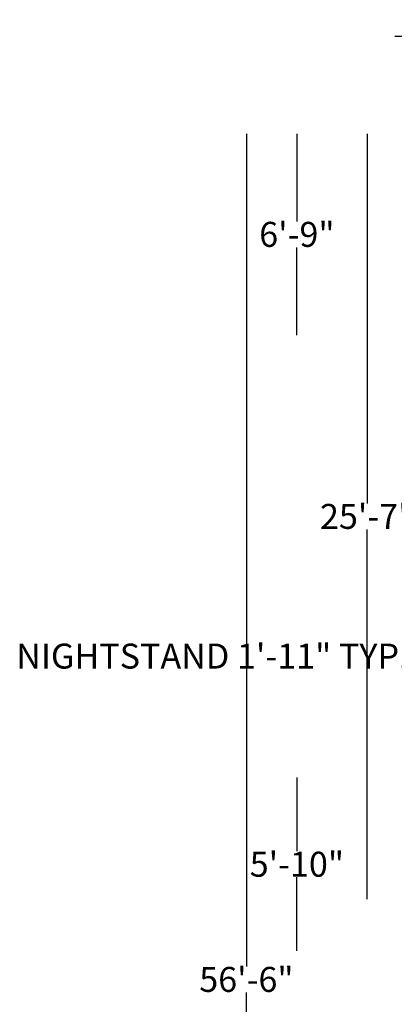
# Model space of a CAD drawing. Units: inches. Extents: x 1198 to 8596, y 144 to 930.
# Tile 2 of 5: x 1198 to 1348, y 536 to 930. Entities that reach past the tile are written whole.
import ezdxf

# ---------------------------------------------------------------- set-up
doc = ezdxf.new("R2010")
doc.units = ezdxf.units.IN
doc.header["$MEASUREMENT"] = 0
doc.layers.add('A-ANNO-DIMS', color=7, linetype='Continuous', lineweight=18)
doc.styles.get("Standard").update_dxf_attribs({"font": 'arial.ttf'})
doc.dimstyles.get("Standard").update_dxf_attribs({"dimtxt": 10, "dimasz": 0.18, "dimexe": 0.18, "dimexo": 0.0625, "dimgap": 0.09, "dimtad": 0, "dimtih": 1, "dimtoh": 1, "dimdec": 0, "dimzin": 0, "dimdsep": 46, "dimlunit": 3, "dimtxsty": 'Standard', "dimcen": 0.09, "dimse1": 1, "dimse2": 1, "dimadec": 0, "dimazin": 0, "dimtfac": 1, "dimtdec": 0, "dimtofl": 0, "dimtmove": 0, "dimatfit": 3, "dimfxl": 1, "dimtolj": 1, "dimtzin": 0, "dimarcsym": 0})

# ---------------------------------------------------------------- blocks, each defined once
blk = doc.blocks.new('*D16')
at = {"layer": 'A-ANNO-DIMS', "color": 0, "lineweight": -2, "transparency": 16777216}
for p, q in [((1337.03, 884.72), (1337.03, 736.59)), ((1337.03, 578.08), (1337.03, 726.2))]:
    blk.add_line(p, q, dxfattribs=at)
at = {"layer": 'A-ANNO-DIMS', "color": 0, "transparency": 16777216}
for points in [[(1337, 884.72), (1337.06, 884.72), (1337.03, 884.9)], [(1337, 578.08), (1337.06, 578.08), (1337.03, 577.9)]]:
    blk.add_solid(points, dxfattribs=at)
at = {"layer": 'Defpoints', "color": 0, "transparency": 16777216}
for p in [(1347.89, 884.9), (1337.03, 577.9), (1347.89, 577.9)]:
    blk.add_point(p, dxfattribs=at)
at = {"layer": 'A-ANNO-DIMS', "color": 0, "transparency": 16777216, "insert": (1337.03, 731.4), "char_height": 10, "attachment_point": 5}
blk.add_mtext('\\A1;25\'-7"', dxfattribs=at)
blk = doc.blocks.new('*D17')
at = {"layer": 'A-ANNO-DIMS', "color": 0, "lineweight": -2, "transparency": 16777216}
for p, q in [((1288.75, 884.72), (1288.75, 551.09)), ((1288.75, 207.08), (1288.75, 540.7))]:
    blk.add_line(p, q, dxfattribs=at)
at = {"layer": 'A-ANNO-DIMS', "color": 0, "transparency": 16777216}
for points in [[(1288.72, 884.72), (1288.78, 884.72), (1288.75, 884.9)], [(1288.72, 207.08), (1288.78, 207.08), (1288.75, 206.9)]]:
    blk.add_solid(points, dxfattribs=at)
at = {"layer": 'Defpoints', "color": 0, "transparency": 16777216}
for p in [(1347.89, 884.9), (1288.75, 206.9), (1347.89, 206.9)]:
    blk.add_point(p, dxfattribs=at)
at = {"layer": 'A-ANNO-DIMS', "color": 0, "transparency": 16777216, "insert": (1288.75, 545.9), "char_height": 10, "attachment_point": 5}
blk.add_mtext('\\A1;56\'-6"', dxfattribs=at)
blk = doc.blocks.new('*D28')
at = {"layer": 'A-ANNO-DIMS', "color": 0, "lineweight": -2, "transparency": 16777216}
for p, q in [((1356.89, 675.44), (1356.71, 675.44)), ((1379.78, 675.44), (1357.07, 675.44))]:
    blk.add_line(p, q, dxfattribs=at)
at = {"layer": 'A-ANNO-DIMS', "color": 0, "transparency": 16777216}
for points in [[(1357.07, 675.47), (1357.07, 675.41), (1356.89, 675.44)], [(1379.78, 675.47), (1379.78, 675.41), (1379.96, 675.44)]]:
    blk.add_solid(points, dxfattribs=at)
at = {"layer": 'Defpoints', "color": 0, "transparency": 16777216}
for p in [(1356.89, 678.9), (1379.96, 678.9), (1356.89, 675.44)]:
    blk.add_point(p, dxfattribs=at)
at = {"layer": 'A-ANNO-DIMS', "color": 0, "transparency": 16777216, "insert": (1275.15, 675.44), "char_height": 10, "attachment_point": 5}
blk.add_mtext('\\A1;NIGHTSTAND 1\'-11" TYP.', dxfattribs=at)
blk = doc.blocks.new('*D30')
at = {"layer": 'A-ANNO-DIMS', "color": 0, "lineweight": -2, "transparency": 16777216}
for p, q in [((1348.07, 923.85), (1374.98, 923.85)), ((1428.71, 923.85), (1401.79, 923.85))]:
    blk.add_line(p, q, dxfattribs=at)
at = {"layer": 'A-ANNO-DIMS', "color": 0, "transparency": 16777216}
for points in [[(1348.07, 923.88), (1348.07, 923.82), (1347.89, 923.85)], [(1428.71, 923.88), (1428.71, 923.82), (1428.89, 923.85)]]:
    blk.add_solid(points, dxfattribs=at)
at = {"layer": 'Defpoints', "color": 0, "transparency": 16777216}
for p in [(1428.89, 923.85), (1347.89, 884.9), (1428.89, 884.9)]:
    blk.add_point(p, dxfattribs=at)
at = {"layer": 'A-ANNO-DIMS', "color": 0, "transparency": 16777216, "insert": (1388.39, 923.85), "char_height": 10, "attachment_point": 5}
blk.add_mtext('\\A1;6\'-9"', dxfattribs=at)
blk = doc.blocks.new('*D36')
at = {"layer": 'A-ANNO-DIMS', "color": 0, "lineweight": -2, "transparency": 16777216}
for p, q in [((1308.94, 884.72), (1308.94, 849.59)), ((1308.94, 804.08), (1308.94, 839.2))]:
    blk.add_line(p, q, dxfattribs=at)
at = {"layer": 'A-ANNO-DIMS', "color": 0, "transparency": 16777216}
for points in [[(1308.91, 884.72), (1308.97, 884.72), (1308.94, 884.9)], [(1308.91, 804.08), (1308.97, 804.08), (1308.94, 803.9)]]:
    blk.add_solid(points, dxfattribs=at)
at = {"layer": 'Defpoints', "color": 0, "transparency": 16777216}
for p in [(1347.89, 884.9), (1308.94, 803.9), (1347.89, 803.9)]:
    blk.add_point(p, dxfattribs=at)
at = {"layer": 'A-ANNO-DIMS', "color": 0, "transparency": 16777216, "insert": (1308.94, 844.4), "char_height": 10, "attachment_point": 5}
blk.add_mtext('\\A1;6\'-9"', dxfattribs=at)
blk = doc.blocks.new('*D54')
at = {"layer": 'A-ANNO-DIMS', "color": 0, "lineweight": -2, "transparency": 16777216}
for p, q in [((1308.94, 626.78), (1308.94, 597.25)), ((1308.94, 557.33), (1308.94, 586.85))]:
    blk.add_line(p, q, dxfattribs=at)
at = {"layer": 'A-ANNO-DIMS', "color": 0, "transparency": 16777216}
for points in [[(1308.91, 626.78), (1308.97, 626.78), (1308.94, 626.96)], [(1308.91, 557.33), (1308.97, 557.33), (1308.94, 557.15)]]:
    blk.add_solid(points, dxfattribs=at)
at = {"layer": 'Defpoints', "color": 0, "transparency": 16777216}
for p in [(1308.94, 626.96), (1802.33, 626.96), (1802.33, 557.15)]:
    blk.add_point(p, dxfattribs=at)
at = {"layer": 'A-ANNO-DIMS', "color": 0, "transparency": 16777216, "insert": (1308.94, 592.05), "char_height": 10, "attachment_point": 5}
blk.add_mtext('\\A1;5\'-10"', dxfattribs=at)

msp = doc.modelspace()

# ---------------------------------------------------------------- dimensions: what is measured, and where the dimension line sits
at = {"layer": 'A-ANNO-DIMS'}
dim = msp.add_linear_dim(base=(1428.89, 923.85), p1=(1347.89, 884.9), p2=(1428.89, 884.9), dimstyle='Standard', override={"dimdec": 1, "dimlfac": 1, "dimrnd": 0, "dimzin": 1, "dimdsep": 46, "dimlunit": 4, "dimfrac": 2}, dxfattribs=at)
dim.commit()
dim.dimension.update_dxf_attribs({"geometry": '*D30', "text_midpoint": (1388.39, 923.85)})
for base, p1, p2, override, picture, middle in [((1288.75, 206.9), (1347.89, 884.9), (1347.89, 206.9), {"dimclrd": 0, "dimclre": 0, "dimclrt": 0}, '*D17', (1288.75, 545.9)), ((1308.94, 803.9), (1347.89, 884.9), (1347.89, 803.9), {"dimdec": 1, "dimlfac": 1, "dimrnd": 0, "dimzin": 1, "dimdsep": 46, "dimlunit": 4, "dimfrac": 2}, '*D36', (1308.94, 844.4)), ((1337.03, 577.9), (1347.89, 884.9), (1347.89, 577.9), {"dimclrd": 0, "dimclre": 0, "dimclrt": 0}, '*D16', (1337.03, 731.4)), ((1308.94, 626.96), (1802.33, 557.15), (1802.33, 626.96), {"dimdec": 1, "dimlfac": 1, "dimrnd": 0, "dimzin": 1, "dimdsep": 46, "dimlunit": 4, "dimfrac": 2}, '*D54', (1308.94, 592.05))]:
    dim = msp.add_linear_dim(base=base, p1=p1, p2=p2, angle=90, dimstyle='Standard', override=override, dxfattribs=at)
    dim.commit()
    dim.dimension.update_dxf_attribs({"geometry": picture, "text_midpoint": middle})
dim = msp.add_linear_dim(base=(1356.89, 675.44), p1=(1379.96, 678.9), p2=(1356.89, 678.9), angle=180, text='NIGHTSTAND <> TYP.', dimstyle='Standard', override={"dimdec": 1, "dimlfac": 1, "dimrnd": 0, "dimzin": 1, "dimdsep": 46, "dimlunit": 4, "dimfrac": 2}, dxfattribs=at)
dim.commit()
dim.dimension.update_dxf_attribs({"geometry": '*D28', "text_midpoint": (1275.15, 675.44)})

doc.saveas('drawing.dxf')
